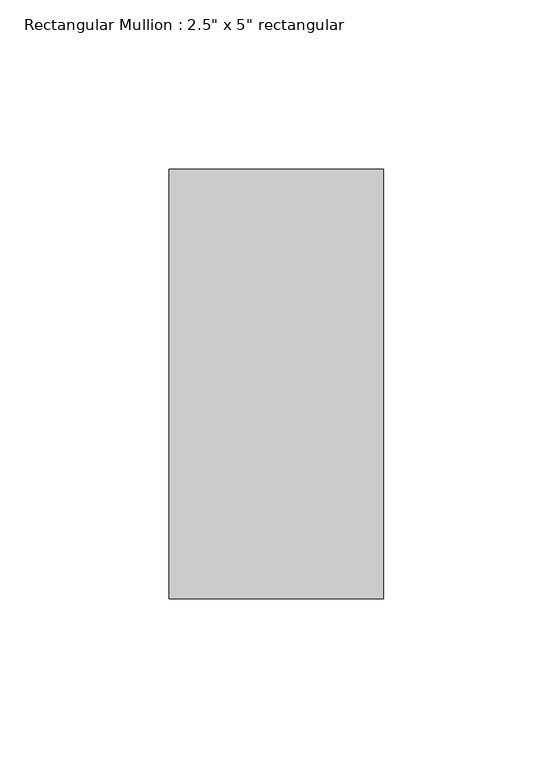
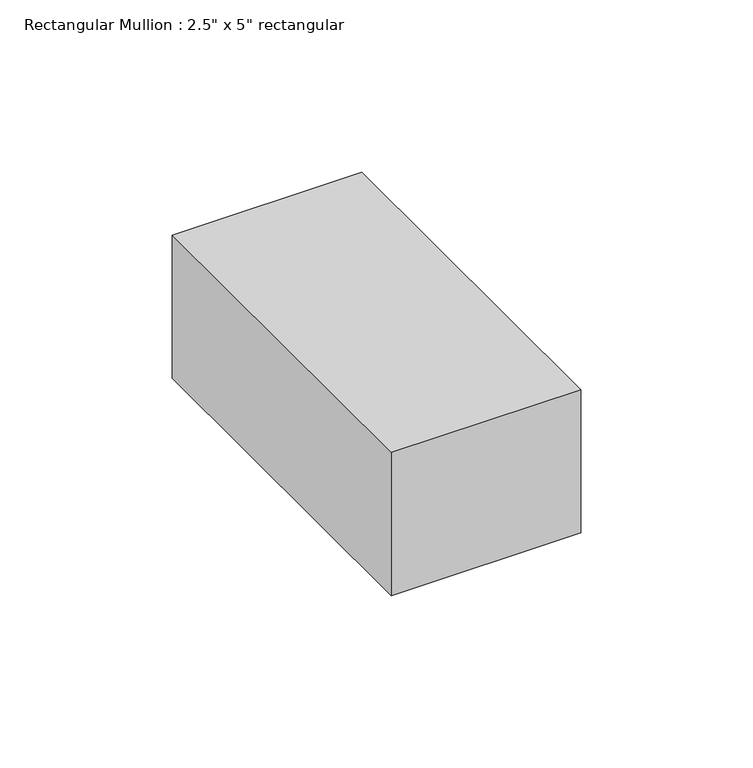
"""IFC4 building model written with IfcOpenShell, lengths in millimetres: member geometry."""

from ifc_helpers import new_model, si_unit, frame, origin, place, context, project, spatial, polyline, outline, extrude, source, transform, mapped, element, save


def member_67d1cd44(model_context):
    return source(origin(), model_context, "Body", "SweptSolid", [
        extrude(outline(polyline([(0.0, 63.5), (0.0, -63.5), (-63.5, -63.5), (-63.5, 63.5), (0.0, 63.5)])), frame((0.0, 0.0, -50.8), z_axis=(0.0, 0.0, 1.0), x_axis=(1.0, 0.0, 0.0)), (0.0, 0.0, 1.0), 50.8),
    ])


if __name__ == "__main__":
    model = new_model("IFC4")
    model_context = context("Model", 3, world=origin())
    ifc_project = project(units=[si_unit("LENGTHUNIT", "METRE", prefix="MILLI")], contexts=[model_context])
    site = spatial("IfcSite", under=ifc_project)
    building = spatial("IfcBuilding", under=site)
    placement = place(None, origin())
    member_shape = member_67d1cd44(model_context)
    element("IfcMember", 1, ObjectType="Rectangular Mullion : 2.5\" x 5\" rectangular", at=placement, inside=building, context=model_context, shape_type="MappedRepresentation", body=[
        mapped(member_shape, transform((0.0, 0.0, 0.0), x_axis=(1.0, 0.0, 0.0), y_axis=(0.0, 1.0, 0.0), z_axis=(0.0, 0.0, 1.0))),
    ])
    save(model, "model.ifc")

# Revit data of these elements
# Type "Rectangular Mullion : 2.5\" x 5\" rectangular"
#   built-in parameter 1007304 = 0.416667 (stored number, unit not read)
#   built-in parameter 1007301 = 0.104167 (stored number, unit not read)
#   built-in parameter 1007300 = 0.104167 (stored number, unit not read)
# Element 1 (IfcMember, "Rectangular Mullion : 2.5\" x 5\" rectangular")
#   Materials on its faces: "Aluminum"
# Materials
#   "Aluminum": class "Metal", colour RGB 247 247 247, transparency 0, Description = "Aluminum 6061", Cost = 0
